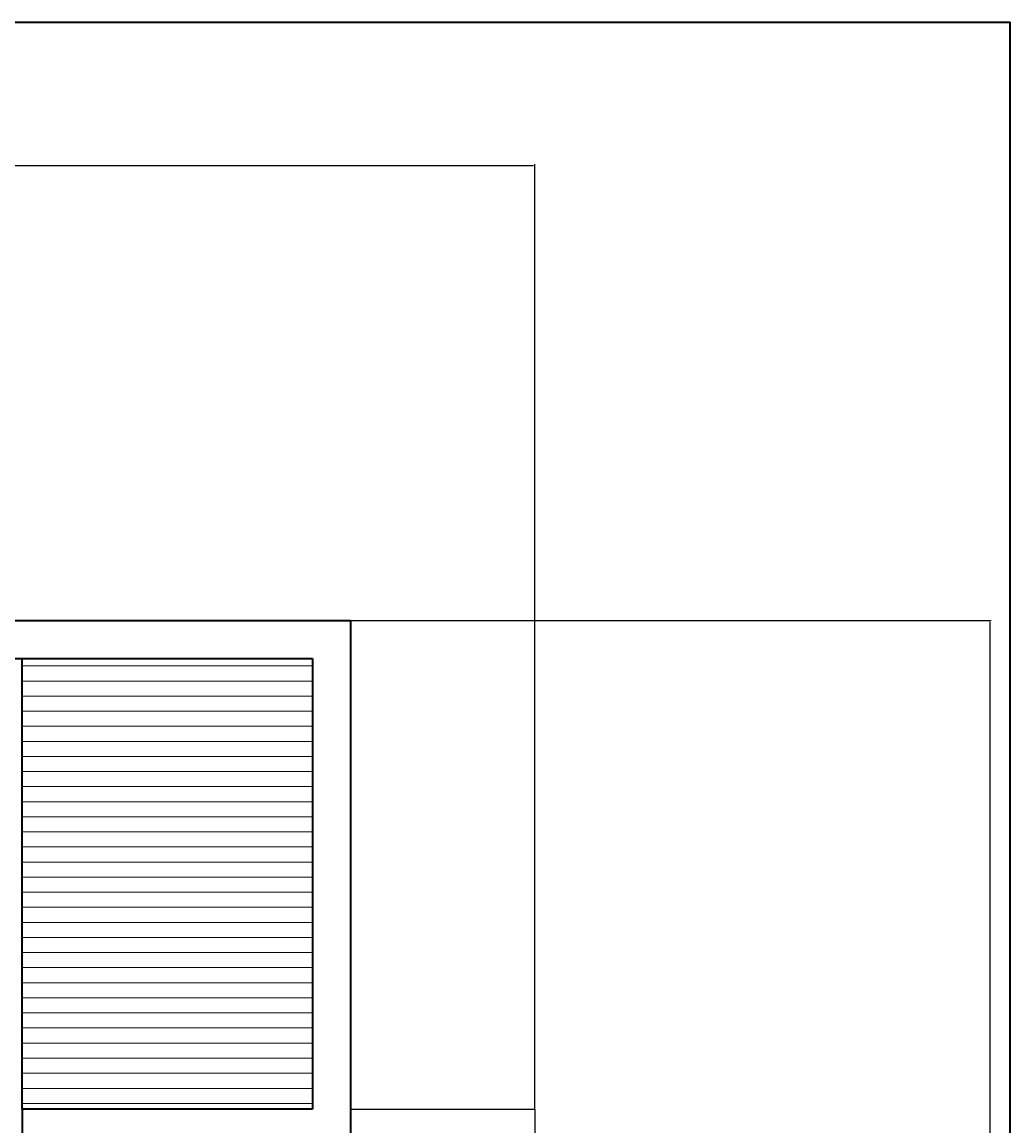
# Model space of a CAD drawing. Units: inches. Extents: x 1088 to 1703, y 668 to 1875.
# Tile 45 of 45: x 1586 to 1703, y 1743 to 1875. Entities that reach past the tile are written whole.
import ezdxf

# ---------------------------------------------------------------- set-up
doc = ezdxf.new("R2010")
doc.units = ezdxf.units.IN
for name, color, linetype, lineweight in [('A-ANNO-DIMS', 2, 'Continuous', 18), ('A-ANNO-TTLB', 7, 'Continuous', 35), ('A-FLOR-HRAL', 7, 'Continuous', 25), ('A-FLOR-PATT', 252, 'Continuous', 13), ('A-WALL', 7, 'Continuous', 35)]:
    doc.layers.add(name, color=color, linetype=linetype, lineweight=lineweight)
doc.styles.get("Standard").update_dxf_attribs({"font": 'arial.ttf'})
doc.dimstyles.get("Standard").update_dxf_attribs({"dimtxt": 0.18, "dimasz": 0.18, "dimexe": 0.18, "dimexo": 0.0625, "dimgap": 0.09, "dimtad": 0, "dimtih": 1, "dimtoh": 1, "dimdec": 4, "dimzin": 0, "dimdsep": 46, "dimtxsty": 'Standard', "dimcen": 0.09, "dimadec": 0, "dimazin": 0, "dimtfac": 1, "dimtdec": 4, "dimtofl": 0, "dimtmove": 0, "dimatfit": 3, "dimfxl": 1, "dimtolj": 1, "dimtzin": 0, "dimarcsym": 0})

# ---------------------------------------------------------------- blocks, each defined once
blk = doc.blocks.new('*D28')
at = {"layer": 'A-ANNO-DIMS', "color": 0, "lineweight": -2, "transparency": 16777216}
for p, q in [((1170.34, 1803.62), (1170.34, 1857.79)), ((1170.52, 1857.61), (1408.15, 1857.61)), ((1646.56, 1857.61), (1408.94, 1857.61)), ((1646.74, 1745.55), (1646.74, 1857.79))]:
    blk.add_line(p, q, dxfattribs=at)
at = {"layer": 'A-ANNO-DIMS', "color": 0, "transparency": 16777216}
for points in [[(1170.52, 1857.64), (1170.52, 1857.58), (1170.34, 1857.61)], [(1646.56, 1857.64), (1646.56, 1857.58), (1646.74, 1857.61)]]:
    blk.add_solid(points, dxfattribs=at)
at = {"layer": 'Defpoints', "color": 0, "transparency": 16777216}
for p in [(1646.74, 1857.61), (1170.34, 1803.56), (1646.74, 1745.49)]:
    blk.add_point(p, dxfattribs=at)
at = {"layer": 'A-ANNO-DIMS', "color": 0, "transparency": 16777216, "insert": (1408.54, 1857.61), "char_height": 0.18, "attachment_point": 5}
blk.add_mtext('\\A1;476.4', dxfattribs=at)
blk = doc.blocks.new('*D30')
at = {"layer": 'A-ANNO-DIMS', "color": 0, "lineweight": -2, "transparency": 16777216}
for p, q in [((1624.91, 1803.56), (1700.97, 1803.56)), ((1700.79, 1803.38), (1700.79, 1609.49)), ((1700.79, 1415.24), (1700.79, 1609.13)), ((1620.41, 1415.06), (1700.97, 1415.06))]:
    blk.add_line(p, q, dxfattribs=at)
at = {"layer": 'A-ANNO-DIMS', "color": 0, "transparency": 16777216}
for points in [[(1700.76, 1803.38), (1700.82, 1803.38), (1700.79, 1803.56)], [(1700.76, 1415.24), (1700.82, 1415.24), (1700.79, 1415.06)]]:
    blk.add_solid(points, dxfattribs=at)
at = {"layer": 'Defpoints', "color": 0, "transparency": 16777216}
for p in [(1624.84, 1803.56), (1700.79, 1803.56), (1620.34, 1415.06)]:
    blk.add_point(p, dxfattribs=at)
at = {"layer": 'A-ANNO-DIMS', "color": 0, "transparency": 16777216, "insert": (1700.79, 1609.31), "char_height": 0.18, "attachment_point": 5}
blk.add_mtext('\\A1;388.5', dxfattribs=at)

msp = doc.modelspace()

# ---------------------------------------------------------------- hatches: boundary and pattern name
at = {"layer": 'A-FLOR-PATT'}
h = msp.add_hatch(dxfattribs=at)
h.set_pattern_fill('ANSI31', color=256, scale=0.564656, angle=-45, style=0)
h.paths.add_polyline_path([(1585.845, 1745.49), (1620.345, 1745.49), (1620.345, 1799.058), (1585.845, 1799.058)])

# ---------------------------------------------------------------- linework, layer by layer
at = {"layer": 'A-ANNO-TTLB'}
msp.add_lwpolyline([(1088.369, 1874.677), (1703.181, 1874.677), (1703.181, 667.947), (1088.369, 667.947)], close=True, dxfattribs=at)
at = {"layer": 'A-FLOR-HRAL'}
for p, q in [((1624.845, 1745.49), (1642.243, 1745.49)), ((1642.243, 1745.49), (1646.743, 1745.49)), ((1646.743, 1745.49), (1646.743, 1474.363))]:
    msp.add_line(p, q, dxfattribs=at)
at = {"layer": 'A-WALL'}
for p, q in [((1437.345, 1803.558), (1624.845, 1803.558)), ((1437.345, 1803.558), (1624.845, 1803.558)), ((1437.345, 1803.558), (1624.845, 1803.558)), ((1437.345, 1803.558), (1624.845, 1803.558)), ((1437.345, 1803.558), (1624.845, 1803.558)), ((1624.845, 1803.558), (1624.845, 1740.99)), ((1441.845, 1799.058), (1620.345, 1799.058)), ((1585.845, 1745.49), (1585.845, 1799.058)), ((1620.345, 1799.058), (1620.345, 1745.49)), ((1585.845, 1745.49), (1585.845, 1736.337)), ((1620.345, 1745.49), (1585.845, 1745.49))]:
    msp.add_line(p, q, dxfattribs=at)

# ---------------------------------------------------------------- dimensions: what is measured, and where the dimension line sits
at = {"layer": 'A-ANNO-DIMS'}
dim = msp.add_linear_dim(base=(1646.743, 1857.608), p1=(1170.345, 1803.558), p2=(1646.743, 1745.49), dimstyle='Standard', override={"dimdec": 1, "dimlfac": 1, "dimrnd": 0, "dimzin": 0, "dimdsep": 46, "dimlunit": 2}, dxfattribs=at)
dim.commit()
dim.dimension.update_dxf_attribs({"geometry": '*D28', "text_midpoint": (1408.544, 1857.608)})
dim = msp.add_linear_dim(base=(1700.793, 1803.558), p1=(1620.345, 1415.058), p2=(1624.845, 1803.558), angle=90, dimstyle='Standard', override={"dimdec": 1, "dimlfac": 1, "dimrnd": 0, "dimzin": 0, "dimdsep": 46, "dimlunit": 2}, dxfattribs=at)
dim.commit()
dim.dimension.update_dxf_attribs({"geometry": '*D30', "text_midpoint": (1700.793, 1609.308)})

doc.saveas('drawing.dxf')
